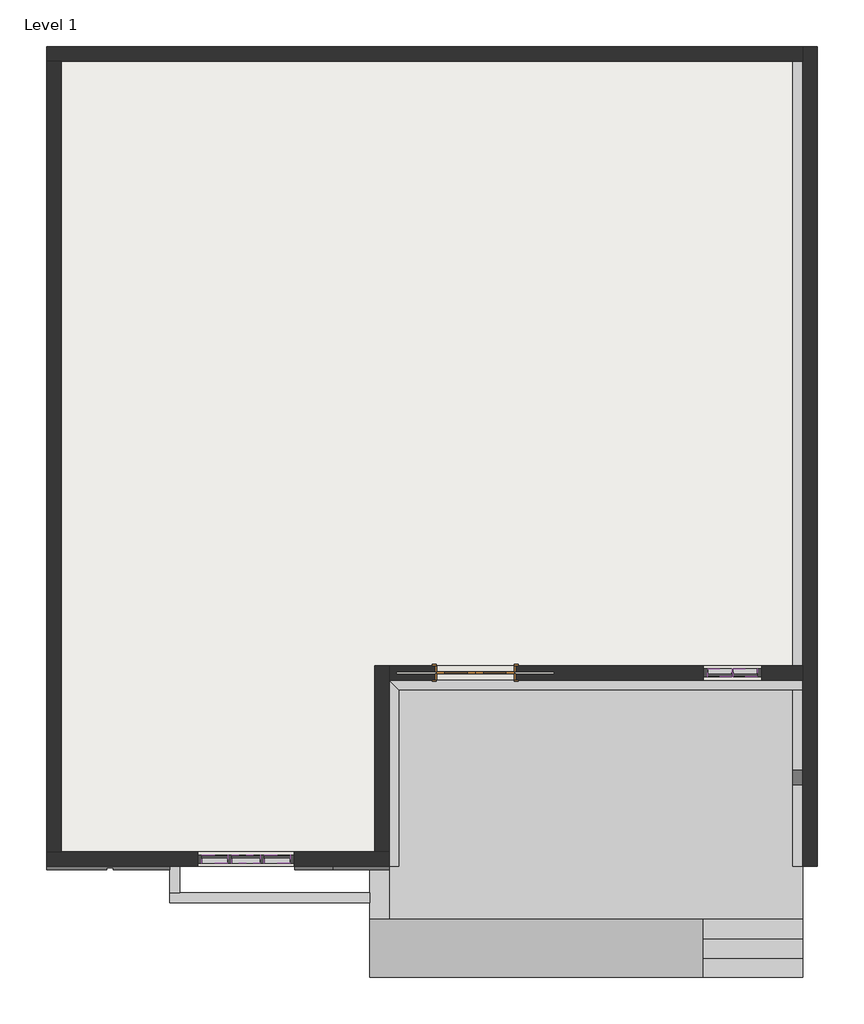
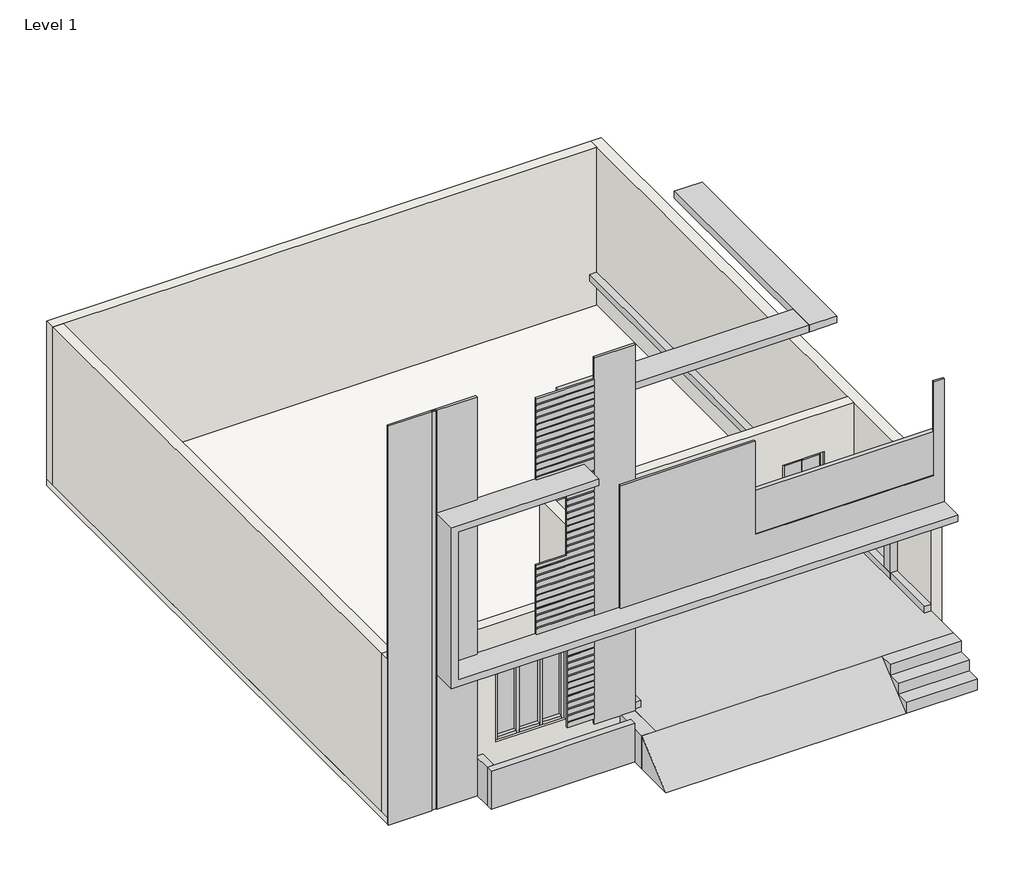
# One storey: 17 members, 6 walls, 5 plates, 4 proxies, 1 door, 1 slab.
"""IFC4 building model written with IfcOpenShell, lengths in millimetres."""

from ifc_helpers import new_model, si_unit, frame, origin, origin_with_axes, place, context, project, spatial, polyline, outline, extrude, faceted_brep, transform, mapped, element, save
from components import generic_models_1_generic_models_1_9d6986c9, generic_models_2_generic_models_2_2375a9c3, door_interior_double_pocket_2_panel_wood_4_x7_3a565322, member_1744d714, member_dc106669, member_d60e8053, member_bc7dbe04, member_2fae0574, member_dfe75557, system_panel_glazed_c73a426b, system_panel_glazed_693f0248, system_panel_glazed_c91192bf

model = new_model("IFC4")

# Units and contexts
model_context = context("Model", 3, world=origin())
ifc_project = project(units=[si_unit("LENGTHUNIT", "METRE", prefix="MILLI")], contexts=[model_context])

# Site, building, storey
site = spatial("IfcSite", under=ifc_project)
building = spatial("IfcBuilding", under=site)
storey = spatial("IfcBuildingStorey", under=building, Name="Level 1", Elevation=0.0)

# Proxies
placement = place(None, origin())
element("IfcBuildingElementProxy", 1, Name="Cornice", ObjectType="Cornice", at=placement, inside=storey, context=model_context, shape_type="SweptSolid", body=[
    extrude(outline(polyline([(1974.9459691, 12882.5033856), (2127.3459691, 12882.5033856), (2127.3459691, 195.2033856), (1974.9459691, 195.2033856), (1974.9459691, 12882.5033856)])), frame((0.0, 0.0, 609.6), z_axis=(0.0, 0.0, 1.0), x_axis=(1.0, 0.0, 0.0)), (0.0, 0.0, 1.0), 152.4),
    extrude(outline(polyline([(-4235.3540309, 195.2033856), (-4387.7540309, 195.2033856), (-4387.7540309, 3128.9033856), (-4235.3540309, 2976.5033856), (-4235.3540309, 195.2033856)])), frame((0.0, 0.0, 609.6), z_axis=(0.0, 0.0, 1.0), x_axis=(1.0, 0.0, 0.0)), (0.0, 0.0, 1.0), 152.4),
])
element("IfcBuildingElementProxy", 2, Name="Cornice", ObjectType="Cornice", at=placement, inside=storey, context=model_context, shape_type="SweptSolid", body=[
    extrude(outline(polyline([(-4235.3540309, 2976.5033856), (-4387.7540309, 3128.9033856), (2127.3459691, 3128.9033856), (2127.3459691, 2976.5033856), (-4235.3540309, 2976.5033856)])), frame((0.0, 0.0, 609.6), z_axis=(0.0, 0.0, 1.0), x_axis=(1.0, 0.0, 0.0)), (0.0, 0.0, 1.0), 152.4),
])
generic_models_1_generic_models_1_shape = generic_models_1_generic_models_1_9d6986c9(model_context)
element("IfcBuildingElementProxy", 3, Name="Generic Models 1 : Generic Models 1", ObjectType="Generic Models 1 : Generic Models 1", at=placement, inside=storey, context=model_context, shape_type="MappedRepresentation", body=[
    mapped(generic_models_1_generic_models_1_shape, transform((0.0, 0.0, 0.0), x_axis=(1.0, 0.0, 0.0), y_axis=(0.0, 1.0, 0.0), z_axis=(0.0, 0.0, 1.0))),
])
generic_models_2_generic_models_2_shape = generic_models_2_generic_models_2_2375a9c3(model_context)
element("IfcBuildingElementProxy", 4, Name="Generic Models 2 : Generic Models 2", ObjectType="Generic Models 2 : Generic Models 2", at=placement, inside=storey, context=model_context, shape_type="MappedRepresentation", body=[
    mapped(generic_models_2_generic_models_2_shape, transform((0.0, 0.0, 0.0), x_axis=(1.0, 0.0, 0.0), y_axis=(0.0, 1.0, 0.0), z_axis=(0.0, 0.0, 1.0))),
])

# Door
door_interior_double_pocket_2_panel_wood_4_x7_shape = door_interior_double_pocket_2_panel_wood_4_x7_3a565322(model_context)
element("IfcDoor", 5, ObjectType="Door-Interior-Double-Pocket-2_Panel-Wood : 4'x7'", at=placement, inside=storey, context=model_context, shape_type="MappedRepresentation", body=[
    mapped(door_interior_double_pocket_2_panel_wood_4_x7_shape, transform((-3028.8540309, 3243.2033856, 609.6), x_axis=(-1.0, 0.0, 0.0), y_axis=(0.0, -1.0, 0.0), z_axis=(0.0, 0.0, 1.0))),
])

# Members
member_shape = member_1744d714(model_context)
element("IfcMember", 6, ObjectType="Rectangular Mullion : 1\" Square", at=placement, inside=storey, context=model_context, shape_type="MappedRepresentation", body=[
    mapped(member_shape, transform((1022.4459691, 3243.2033856, 914.4), x_axis=(-1.0, 0.0, 0.0), y_axis=(0.0, 1.0, 0.0), z_axis=(0.0, 0.0, -1.0))),
])
member_2_shape = member_dc106669(model_context)
element("IfcMember", 7, ObjectType="Rectangular Mullion : 2.5\" x 5\" rectangular", at=placement, inside=storey, context=model_context, shape_type="MappedRepresentation", body=[
    mapped(member_2_shape, transform((-5943.5040309, 309.5033856, 2743.2), x_axis=(0.0, 0.0, 1.0), y_axis=(0.0, -1.0, 0.0), z_axis=(1.0, 0.0, 0.0))),
])
element("IfcMember", 8, ObjectType="Rectangular Mullion : 2.5\" x 5\" rectangular", at=placement, inside=storey, context=model_context, shape_type="MappedRepresentation", body=[
    mapped(member_2_shape, transform((-6927.7540309, 309.5033856, 2743.2), x_axis=(0.0, 0.0, 1.0), y_axis=(0.0, -1.0, 0.0), z_axis=(1.0, 0.0, 0.0))),
])
element("IfcMember", 9, ObjectType="Rectangular Mullion : 2.5\" x 5\" rectangular", at=placement, inside=storey, context=model_context, shape_type="MappedRepresentation", body=[
    mapped(member_2_shape, transform((-7340.5040309, 309.5033856, 914.4), x_axis=(0.0, 0.0, -1.0), y_axis=(0.0, -1.0, 0.0), z_axis=(-1.0, 0.0, 0.0))),
])
element("IfcMember", 10, ObjectType="Rectangular Mullion : 2.5\" x 5\" rectangular", at=placement, inside=storey, context=model_context, shape_type="MappedRepresentation", body=[
    mapped(member_2_shape, transform((-6356.2540309, 309.5033856, 914.4), x_axis=(0.0, 0.0, -1.0), y_axis=(0.0, -1.0, 0.0), z_axis=(-1.0, 0.0, 0.0))),
])
member_3_shape = member_d60e8053(model_context)
element("IfcMember", 11, ObjectType="Rectangular Mullion : 2.5\" x 5\" rectangular", at=placement, inside=storey, context=model_context, shape_type="MappedRepresentation", body=[
    mapped(member_3_shape, transform((-6896.0040309, 309.5033856, 914.4), x_axis=(1.0, 0.0, 0.0), y_axis=(0.0, -1.0, 0.0), z_axis=(0.0, 0.0, -1.0))),
])
element("IfcMember", 12, ObjectType="Rectangular Mullion : 2.5\" x 5\" rectangular", at=placement, inside=storey, context=model_context, shape_type="MappedRepresentation", body=[
    mapped(member_3_shape, transform((-6388.0040309, 309.5033856, 914.4), x_axis=(1.0, 0.0, 0.0), y_axis=(0.0, -1.0, 0.0), z_axis=(0.0, 0.0, -1.0))),
])
member_4_shape = member_bc7dbe04(model_context)
element("IfcMember", 13, ObjectType="Rectangular Mullion : 2.5\" x 5\" rectangular", at=placement, inside=storey, context=model_context, shape_type="MappedRepresentation", body=[
    mapped(member_4_shape, transform((-6864.2540309, 309.5033856, 914.4), x_axis=(0.0, 0.0, -1.0), y_axis=(0.0, -1.0, 0.0), z_axis=(-1.0, 0.0, 0.0))),
])
element("IfcMember", 14, ObjectType="Rectangular Mullion : 2.5\" x 5\" rectangular", at=placement, inside=storey, context=model_context, shape_type="MappedRepresentation", body=[
    mapped(member_4_shape, transform((-6419.7540309, 309.5033856, 2743.2), x_axis=(0.0, 0.0, 1.0), y_axis=(0.0, -1.0, 0.0), z_axis=(1.0, 0.0, 0.0))),
])
member_5_shape = member_2fae0574(model_context)
element("IfcMember", 15, ObjectType="Rectangular Mullion : 2.5\" x 5\" rectangular", at=placement, inside=storey, context=model_context, shape_type="MappedRepresentation", body=[
    mapped(member_5_shape, transform((-7404.0040309, 309.5033856, 2743.2), x_axis=(-1.0, 0.0, 0.0), y_axis=(0.0, -1.0, 0.0), z_axis=(0.0, 0.0, 1.0))),
])
element("IfcMember", 16, ObjectType="Rectangular Mullion : 2.5\" x 5\" rectangular", at=placement, inside=storey, context=model_context, shape_type="MappedRepresentation", body=[
    mapped(member_5_shape, transform((1479.6459691, 3243.2033856, 2743.2), x_axis=(1.0, 0.0, 0.0), y_axis=(0.0, 1.0, 0.0), z_axis=(0.0, 0.0, 1.0))),
])
element("IfcMember", 17, ObjectType="Rectangular Mullion : 2.5\" x 5\" rectangular", at=placement, inside=storey, context=model_context, shape_type="MappedRepresentation", body=[
    mapped(member_5_shape, transform((-5880.0040309, 309.5033856, 914.4), x_axis=(1.0, 0.0, 0.0), y_axis=(0.0, -1.0, 0.0), z_axis=(0.0, 0.0, -1.0))),
])
element("IfcMember", 18, ObjectType="Rectangular Mullion : 2.5\" x 5\" rectangular", at=placement, inside=storey, context=model_context, shape_type="MappedRepresentation", body=[
    mapped(member_5_shape, transform((565.2459691, 3243.2033856, 914.4), x_axis=(-1.0, 0.0, 0.0), y_axis=(0.0, 1.0, 0.0), z_axis=(0.0, 0.0, -1.0))),
])
member_6_shape = member_dfe75557(model_context)
element("IfcMember", 19, ObjectType="Rectangular Mullion : 2.5\" x 5\" rectangular", at=placement, inside=storey, context=model_context, shape_type="MappedRepresentation", body=[
    mapped(member_6_shape, transform((628.7459691, 3243.2033856, 2743.2), x_axis=(0.0, 0.0, 1.0), y_axis=(0.0, 1.0, 0.0), z_axis=(-1.0, 0.0, 0.0))),
])
element("IfcMember", 20, ObjectType="Rectangular Mullion : 2.5\" x 5\" rectangular", at=placement, inside=storey, context=model_context, shape_type="MappedRepresentation", body=[
    mapped(member_6_shape, transform((1035.1459691, 3243.2033856, 2743.2), x_axis=(0.0, 0.0, 1.0), y_axis=(0.0, 1.0, 0.0), z_axis=(-1.0, 0.0, 0.0))),
])
element("IfcMember", 21, ObjectType="Rectangular Mullion : 2.5\" x 5\" rectangular", at=placement, inside=storey, context=model_context, shape_type="MappedRepresentation", body=[
    mapped(member_6_shape, transform((1416.1459691, 3243.2033856, 914.4), x_axis=(0.0, 0.0, -1.0), y_axis=(0.0, 1.0, 0.0), z_axis=(1.0, 0.0, 0.0))),
])
element("IfcMember", 22, ObjectType="Rectangular Mullion : 2.5\" x 5\" rectangular", at=placement, inside=storey, context=model_context, shape_type="MappedRepresentation", body=[
    mapped(member_6_shape, transform((1009.7459691, 3243.2033856, 914.4), x_axis=(0.0, 0.0, -1.0), y_axis=(0.0, 1.0, 0.0), z_axis=(1.0, 0.0, 0.0))),
])

# Plates
system_panel_glazed_shape = system_panel_glazed_c73a426b(model_context)
element("IfcPlate", 23, ObjectType="System Panel : Glazed", at=placement, inside=storey, context=model_context, shape_type="MappedRepresentation", body=[
    mapped(system_panel_glazed_shape, transform((-7134.1290309, 309.5033856, 977.9), x_axis=(1.0, 0.0, 0.0), y_axis=(0.0, 1.0, 0.0), z_axis=(0.0, 0.0, 1.0))),
])
element("IfcPlate", 24, ObjectType="System Panel : Glazed", at=placement, inside=storey, context=model_context, shape_type="MappedRepresentation", body=[
    mapped(system_panel_glazed_shape, transform((-6149.8790309, 309.5033856, 977.9), x_axis=(1.0, 0.0, 0.0), y_axis=(0.0, 1.0, 0.0), z_axis=(0.0, 0.0, 1.0))),
])
system_panel_glazed_2_shape = system_panel_glazed_693f0248(model_context)
element("IfcPlate", 25, ObjectType="System Panel : Glazed", at=placement, inside=storey, context=model_context, shape_type="MappedRepresentation", body=[
    mapped(system_panel_glazed_2_shape, transform((-6642.0040309, 309.5033856, 977.9), x_axis=(1.0, 0.0, 0.0), y_axis=(0.0, 1.0, 0.0), z_axis=(0.0, 0.0, 1.0))),
])
system_panel_glazed_3_shape = system_panel_glazed_c91192bf(model_context)
element("IfcPlate", 26, ObjectType="System Panel : Glazed", at=placement, inside=storey, context=model_context, shape_type="MappedRepresentation", body=[
    mapped(system_panel_glazed_3_shape, transform((1219.2959691, 3243.2033856, 977.9), x_axis=(-1.0, 0.0, 0.0), y_axis=(0.0, -1.0, 0.0), z_axis=(0.0, 0.0, 1.0))),
])
element("IfcPlate", 27, ObjectType="System Panel : Glazed", at=placement, inside=storey, context=model_context, shape_type="MappedRepresentation", body=[
    mapped(system_panel_glazed_3_shape, transform((825.5959691, 3243.2033856, 977.9), x_axis=(-1.0, 0.0, 0.0), y_axis=(0.0, -1.0, 0.0), z_axis=(0.0, 0.0, 1.0))),
])

# Slab
element("IfcSlab", 28, ObjectType="6\"", at=placement, inside=storey, context=model_context, shape_type="SweptSolid", body=[
    extrude(outline(polyline([(-9785.2540309, 13111.1033856), (2355.9459691, 13111.1033856), (2355.9459691, 195.2033856), (2127.3459691, 195.2033856), (2127.3459691, 3128.9033856), (-4387.7540309, 3128.9033856), (-4387.7540309, 195.2033856), (-9785.2540309, 195.2033856), (-9785.2540309, 13111.1033856)])), frame((0.0, 0.0, -152.4), z_axis=(0.0, 0.0, 1.0), x_axis=(1.0, 0.0, 0.0)), (0.0, 0.0, 1.0), 152.4),
])

# Walls
element("IfcWall", 29, ObjectType="9\" wall", at=placement, inside=storey, context=model_context, shape_type="Brep", body=[
    faceted_brep([(-9785.2540309, 12882.5033856, 0.0), (-9556.6540309, 12882.5033856, 0.0), (2127.3459691, 12882.5033856, 0.0), (2127.3459691, 12882.5033856, 3657.6), (-9556.6540309, 12882.5033856, 3657.6), (-9785.2540309, 12882.5033856, 3657.6), (-9785.2540309, 13111.1033856, 0.0), (-9785.2540309, 13111.1033856, 3657.6), (2127.3459691, 13111.1033856, 3657.6), (2127.3459691, 13111.1033856, 0.0)], [[[0, 1, 2, 3, 4, 5]], [[6, 7, 8, 9]], [[2, 1, 0, 6, 9]], [[5, 4, 3, 8, 7]], [[0, 5, 7, 6]], [[3, 2, 9, 8]]]),
])
element("IfcWall", 30, ObjectType="9\" wall", at=placement, inside=storey, context=model_context, shape_type="Brep", body=[
    faceted_brep([(2127.3459691, 13111.1033856, 0.0), (2127.3459691, 12882.5033856, 0.0), (2127.3459691, 3357.5033856, 0.0), (2127.3459691, 3128.9033856, 0.0), (2127.3459691, 195.2033856, 0.0), (2127.3459691, 195.2033856, 3657.6), (2127.3459691, 3128.9033856, 3657.6), (2127.3459691, 3357.5033856, 3657.6), (2127.3459691, 12882.5033856, 3657.6), (2127.3459691, 13111.1033856, 3657.6), (2355.9459691, 13111.1033856, 0.0), (2355.9459691, 13111.1033856, 3657.6), (2355.9459691, 195.2033856, 3657.6), (2355.9459691, 195.2033856, 0.0)], [[[0, 1, 2, 3, 4, 5, 6, 7, 8, 9]], [[10, 11, 12, 13]], [[4, 3, 2, 1, 0, 10, 13]], [[5, 4, 13, 12]], [[9, 8, 7, 6, 5, 12, 11]], [[0, 9, 11, 10]]]),
])
element("IfcWall", 31, ObjectType="9\" wall", at=placement, inside=storey, context=model_context, shape_type="Brep", body=[
    faceted_brep([(-4387.7540309, 3128.9033856, 0.0), (2127.3459691, 3128.9033856, 0.0), (2127.3459691, 3128.9033856, 3657.6), (-4387.7540309, 3128.9033856, 3657.6), (-3663.8540309, 3128.9033856, 2768.6), (-2393.8540309, 3128.9033856, 2768.6), (-2393.8540309, 3128.9033856, 609.6), (-3663.8540309, 3128.9033856, 609.6), (1479.6459691, 3128.9033856, 2743.2), (1479.6459691, 3128.9033856, 914.4), (565.2459691, 3128.9033856, 914.4), (565.2459691, 3128.9033856, 2743.2), (2127.3459691, 3357.5033856, 0.0), (-4387.7540309, 3357.5033856, 0.0), (-4387.7540309, 3357.5033856, 3657.6), (2127.3459691, 3357.5033856, 3657.6), (-2393.8540309, 3357.5033856, 2768.6), (-3663.8540309, 3357.5033856, 2768.6), (-3663.8540309, 3357.5033856, 609.6), (-2393.8540309, 3357.5033856, 609.6), (1479.6459691, 3357.5033856, 914.4), (1479.6459691, 3357.5033856, 2743.2), (565.2459691, 3357.5033856, 2743.2), (565.2459691, 3357.5033856, 914.4), (-4273.4540309, 3222.5658856, 2768.6), (-4273.4540309, 3263.8408856, 2768.6), (-3663.8540309, 3263.8408856, 2768.6), (-2393.8540309, 3263.8408856, 2768.6), (-1784.2540309, 3263.8408856, 2768.6), (-1784.2540309, 3222.5658856, 2768.6), (-2393.8540309, 3222.5658856, 2768.6), (-3663.8540309, 3222.5658856, 2768.6), (-4273.4540309, 3222.5658856, 609.6), (-3663.8540309, 3222.5658856, 609.6), (-2393.8540309, 3222.5658856, 609.6), (-1784.2540309, 3222.5658856, 609.6), (-1784.2540309, 3263.8408856, 609.6), (-2393.8540309, 3263.8408856, 609.6), (-3663.8540309, 3263.8408856, 609.6), (-4273.4540309, 3263.8408856, 609.6)], [[[0, 1, 2, 3], [4, 5, 6, 7], [8, 9, 10, 11]], [[12, 13, 14, 15], [16, 17, 18, 19], [20, 21, 22, 23]], [[1, 0, 13, 12]], [[3, 2, 15, 14]], [[0, 3, 14, 13]], [[2, 1, 12, 15]], [[24, 25, 26, 17, 16, 27, 28, 29, 30, 5, 4, 31]], [[32, 33, 7, 6, 34, 35, 36, 37, 19, 18, 38, 39]], [[24, 31, 33, 32]], [[31, 4, 7, 33]], [[5, 30, 34, 6]], [[30, 29, 35, 34]], [[29, 28, 36, 35]], [[28, 27, 37, 36]], [[27, 16, 19, 37]], [[17, 26, 38, 18]], [[26, 25, 39, 38]], [[25, 24, 32, 39]], [[8, 21, 20, 9]], [[21, 8, 11, 22]], [[22, 11, 10, 23]], [[9, 20, 23, 10]]]),
])
element("IfcWall", 32, ObjectType="9\" wall", at=placement, inside=storey, context=model_context, shape_type="Brep", body=[
    faceted_brep([(-4387.7540309, 423.8033856, 0.0), (-4616.3540309, 423.8033856, 0.0), (-9556.6540309, 423.8033856, 0.0), (-9785.2540309, 423.8033856, 0.0), (-9785.2540309, 423.8033856, 3657.6), (-9556.6540309, 423.8033856, 3657.6), (-4616.3540309, 423.8033856, 3657.6), (-4387.7540309, 423.8033856, 3657.6), (-7404.0040309, 423.8033856, 2743.2), (-7404.0040309, 423.8033856, 914.4), (-5880.0040309, 423.8033856, 914.4), (-5880.0040309, 423.8033856, 2743.2), (-9785.2540309, 195.2033856, 0.0), (-4387.7540309, 195.2033856, 0.0), (-4387.7540309, 195.2033856, 3657.6), (-9785.2540309, 195.2033856, 3657.6), (-7404.0040309, 195.2033856, 914.4), (-7404.0040309, 195.2033856, 2743.2), (-5880.0040309, 195.2033856, 2743.2), (-5880.0040309, 195.2033856, 914.4)], [[[0, 1, 2, 3, 4, 5, 6, 7], [8, 9, 10, 11]], [[12, 13, 14, 15], [16, 17, 18, 19]], [[3, 2, 1, 0, 13, 12]], [[7, 6, 5, 4, 15, 14]], [[4, 3, 12, 15]], [[0, 7, 14, 13]], [[16, 9, 8, 17]], [[17, 8, 11, 18]], [[18, 11, 10, 19]], [[9, 16, 19, 10]]]),
])
element("IfcWall", 33, ObjectType="9\" wall", at=placement, inside=storey, context=model_context, shape_type="SweptSolid", body=[
    extrude(outline(polyline([(-9556.6540309, 12882.5033856), (-9556.6540309, 423.8033856), (-9785.2540309, 423.8033856), (-9785.2540309, 12882.5033856), (-9556.6540309, 12882.5033856)])), origin_with_axes(), (0.0, 0.0, 1.0), 3657.6),
])
element("IfcWall", 34, ObjectType="9\" wall", at=placement, inside=storey, context=model_context, shape_type="Brep", body=[
    faceted_brep([(-4387.7540309, 423.8033856, 0.0), (-4387.7540309, 3128.9033856, 0.0), (-4387.7540309, 3357.5033856, 0.0), (-4387.7540309, 3357.5033856, 3657.6), (-4387.7540309, 3128.9033856, 3657.6), (-4387.7540309, 423.8033856, 3657.6), (-4616.3540309, 423.8033856, 0.0), (-4616.3540309, 423.8033856, 3657.6), (-4616.3540309, 3357.5033856, 3657.6), (-4616.3540309, 3357.5033856, 0.0)], [[[0, 1, 2, 3, 4, 5]], [[6, 7, 8, 9]], [[2, 1, 0, 6, 9]], [[5, 4, 3, 8, 7]], [[3, 2, 9, 8]], [[0, 5, 7, 6]]]),
])

save(model, "model.ifc")

# Revit data of these elements
# Type "Door-Interior-Double-Pocket-2_Panel-Wood : 4'x7'"
#   Type Mark = "9"
#   Assembly Code = "C1020300"
#   Analytic Construction = "Wooden"
#   Top Rail = 0' - 4 11/16"
#   Thickness = 0' - 1 3/8"
#   Thermal Resistance (R) = 2.5876 (h·ft²·°F)/BTU
#   Stiles = 0' - 4 3/4"
#   Rough Width = 8' - 2"
#   Rough Height = 7' - 4 1/2"
#   Panel Width = 2' - 0"
#   Lock Rail = 0' - 7 1/2"
#   Location [instance default] = 2' - 1"
#   Height = 7' - 0"
#   Width = 4' - 0"
#   Heat Transfer Coefficient (U) = 0.3865 BTU/(h·ft²·°F)
#   Bottom Rail = 0' - 9 1/8"
#   Panel Open [instance default] = no
#   Trim Material = Cherry
#   Panel Material = Cherry
#   Frame Material = Cherry
#   Visual Light Transmittance = 0
#   Solar Heat Gain Coefficient = 0
#   Wall Closure = (empty or 0)
#   Function = (empty or 0)
# Type "Rectangular Mullion : 1\" Square"
#   built-in parameter 1007304 = 0.0833333 (stored number, unit not read)
#   built-in parameter 1007301 = 0.0416667 (stored number, unit not read)
#   built-in parameter 1007300 = 0.0416667 (stored number, unit not read)
# Type "Rectangular Mullion : 2.5\" x 5\" rectangular"
#   built-in parameter 1007304 = 0.416667 (stored number, unit not read)
#   built-in parameter 1007301 = 0.104167 (stored number, unit not read)
#   built-in parameter 1007300 = 0.104167 (stored number, unit not read)
# Type "System Panel : Glazed"
#   Construction Type Id = "GSP4R"
#   Analytic Construction = "1/8 in Pilkington single glazing"
#   Visual Light Transmittance = 0.9
#   Solar Heat Gain Coefficient = 0.86
#   Heat Transfer Coefficient (U) = 1.18115 BTU/(h·ft²·°F)
#   Define Thermal Properties by = 1
# Type "6\""
#   Assembly Code = "B1010"
#   Function = 0
#   Layers, outside or top first: 0' - 6" "Gypsum Wall Board" (function 1)
# Type "9\" wall"
#   Assembly Code = "B2010"
#   Layers, outside or top first: 0' - 9" "Gypsum Wall Board" (function 1)
# Elements 1, 2 (IfcBuildingElementProxy, "Cornice")
#   Phase Created = New Construction
# Element 3 (IfcBuildingElementProxy, "Generic Models 1 : Generic Models 1")
#   Phase Created = New Construction
#   Materials on its faces: "Gypsum Wall Board", "Gravel"
# Element 4 (IfcBuildingElementProxy, "Generic Models 2 : Generic Models 2")
#   Phase Created = New Construction
#   Materials on its faces: "Gypsum Wall Board", "Laminate, Ivory, Matte"
# Element 5 (IfcDoor, "Door-Interior-Double-Pocket-2_Panel-Wood : 4'x7'")
#   Location = 2' - 1"
#   Panel Open = no
#   Phase Created = New Construction
#   Materials on its faces: "Cherry"
# Element 6 (IfcMember, "Rectangular Mullion : 1\" Square")
#   Phase Created = New Construction
#   Materials on its faces: "Aluminum"
# Elements 7, 8, 9, 10, 11, 12, 13, 14, 15, 16, 17, 18, 19, 20, 21, 22 (IfcMember, "Rectangular Mullion : 2.5\" x 5\" rectangular")
#   Phase Created = New Construction
# Elements 23, 24, 25, 26, 27 (IfcPlate, "System Panel : Glazed")
#   Phase Created = New Construction
#   Materials on its faces: "Glass"
# Element 28 (IfcSlab, "6\"")
#   built-in parameter 1001955 = 3.14159 (stored number, unit not read)
#   Height Offset From Level = 0' - 0"
#   Phase Created = New Construction
#   Materials on its faces: "Gypsum Wall Board"
# Elements 29, 30, 31, 32, 33, 34 (IfcWall, "9\" wall")
#   Top Offset = 0' - 0"
#   Base Offset = 0' - 0"
#   wall height = 12' - 0"
#   Phase Created = New Construction
#   Base Constraint = Level 1
#   Top Constraint = Level 2
#   Materials on its faces: "Gypsum Wall Board"
# Materials
#   "Cherry": class "Wood", colour RGB 226 177 128, transparency 0, Description = "Prunus Serotina", Cost = 0
#   "Gypsum Wall Board": class "Generic", colour RGB 127 127 127, transparency 0, Description = "Gypsum Wall Board", Cost = 0
#   "Gravel": class "Generic", colour RGB 120 120 120, transparency 0, Description = "Crushed stone or gravel", Cost = 0
#   "Laminate, Ivory, Matte": class "Plastic", colour RGB 247 247 239, transparency 0, Description = "Plastic Laminate - Ivory, Matte", Cost = 0
#   "Aluminum": class "Metal", colour RGB 247 247 247, transparency 0, Description = "Aluminum 6061", Cost = 0
#   "Glass": class "Glass", colour RGB 0 128 192, transparency 0.75, Description = "Soda Lime Glass", Cost = 0
